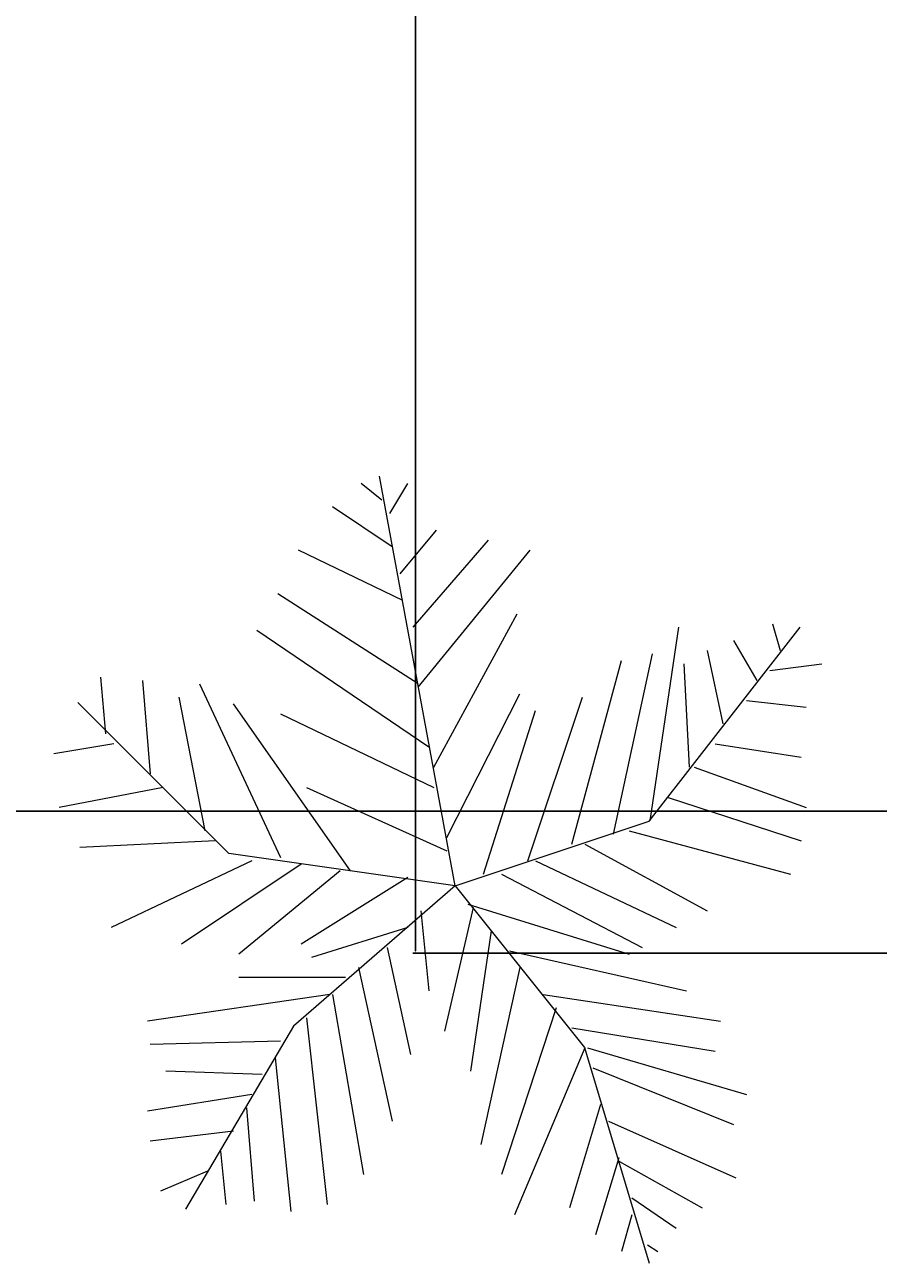
# Model space of a CAD drawing. Units: inches. Extents: x -301 to 715, y -607 to 364.
# Tile 92 of 141: x 134 to 194, y -256 to -168. Entities that reach past the tile are written whole.
import ezdxf

# ---------------------------------------------------------------- set-up
doc = ezdxf.new("R2010")
doc.units = ezdxf.units.IN
doc.header["$MEASUREMENT"] = 0
doc.layers.add('A-ANNO-DIMS', color=2, linetype='Continuous', lineweight=18)
doc.layers.add('L-PLNT', color=94, linetype='Continuous', lineweight=13)
doc.styles.get("Standard").update_dxf_attribs({"font": 'arial.ttf'})
doc.dimstyles.get("Standard").update_dxf_attribs({"dimtxt": 0.18, "dimasz": 0.18, "dimexe": 0.18, "dimexo": 0.0625, "dimgap": 0.09, "dimtad": 0, "dimtih": 1, "dimtoh": 1, "dimdec": 1, "dimzin": 0, "dimdsep": 46, "dimlunit": 4, "dimtxsty": 'Standard', "dimcen": 0.09, "dimclrd": 3, "dimclre": 4, "dimclrt": 6, "dimadec": 0, "dimazin": 0, "dimtfac": 1, "dimtdec": 1, "dimtofl": 0, "dimtmove": 0, "dimatfit": 3, "dimfxl": 1, "dimtfill": 2, "dimtfillclr": 51, "dimtolj": 1, "dimtzin": 0, "dimarcsym": 0})

# ---------------------------------------------------------------- blocks, each defined once
blk = doc.blocks.new('*U33')
for p, q in [((0, 0), (-10.5, 57)), ((-10.186, 53.64), (-13.084, 55.962)), ((-9.099, 51.782), (-6.563, 55.962)), ((-8.737, 47.138), (-17.069, 52.711)), ((-7.65, 43.423), (-2.578, 49.46)), ((-7.288, 39.707), (-21.778, 46.673)), ((-5.839, 35.992), (4.667, 48.067)), ((-5.114, 27.632), (10.463, 46.673)), ((-5.114, 28.097), (-24.676, 40.636)), ((-2.941, 16.486), (8.652, 37.85)), ((44.153, 36.456), (45.239, 32.741)), ((-3.665, 19.273), (-27.574, 35.527)), ((27, 9), (48, 36)), ((27.127, 9.056), (31.112, 35.992)), ((35.096, 32.741), (37.27, 22.524)), ((38.719, 34.134), (41.979, 28.561)), ((16.259, 5.805), (23.142, 31.348)), ((22.055, 7.198), (27.489, 32.277)), ((31.836, 30.883), (32.561, 16.486)), ((43.791, 29.954), (51.036, 30.883)), ((-48.585, 21.131), (-49.309, 29.026)), ((-43.513, 28.561), (-42.427, 15.558)), ((-35.544, 28.097), (-24.314, 3.947)), ((-38.442, 26.239), (-34.819, 7.663)), ((-1.129, 6.734), (9.014, 26.704)), ((10.101, 3.483), (17.708, 26.239)), ((-31.5, 4.5), (-52.5, 25.5)), ((-14.533, 2.09), (-30.834, 25.31)), ((3.942, 1.625), (11.187, 24.381)), ((40.53, 25.775), (48.862, 24.846)), ((-24.314, 23.917), (-2.941, 13.7)), ((-47.498, 19.737), (-55.83, 18.344)), ((36.183, 19.737), (48.137, 17.88)), ((33.285, 16.486), (48.862, 10.913)), ((-40.615, 13.7), (-55.105, 10.913)), ((-20.691, 13.7), (-1.129, 4.876)), ((29.662, 12.307), (48.137, 6.269)), ((0, 0), (27, 9)), ((24.229, 7.663), (46.688, 1.625)), ((-33.37, 6.269), (-52.207, 5.34)), ((18.07, 5.805), (35.096, -3.483)), ((-28.299, 3.483), (-47.86, -5.805)), ((0, 0), (-31.5, 4.5)), ((11.187, 3.483), (30.749, -5.805)), ((-21.416, 3.018), (-38.079, -8.128)), ((-15.982, 2.09), (-30.11, -9.521)), ((0, 0), (-22.5, -19.5)), ((-6.563, 1.161), (-21.416, -8.128)), ((0, 0), (18, -22.5)), ((6.478, 1.625), (26.04, -8.592)), ((2.493, -3.019), (-1.491, -20.202)), ((1.769, -2.555), (24.229, -9.521)), ((-4.752, -3.483), (-3.665, -14.629)), ((-6.563, -5.805), (-19.967, -9.985)), ((5.029, -6.27), (2.131, -25.775)), ((-9.461, -8.592), (-6.201, -23.453)), ((7.565, -9.056), (32.198, -14.629)), ((-13.446, -11.378), (-8.737, -32.741)), ((9.014, -11.378), (3.58, -35.992)), ((-15.257, -12.772), (-30.11, -12.772)), ((-17.431, -15.094), (-42.789, -18.809)), ((-17.069, -15.094), (-12.721, -40.172)), ((12.274, -15.094), (36.907, -18.809)), ((14.085, -16.951), (6.478, -40.172)), ((-20.691, -18.345), (-17.793, -44.352)), ((-22.5, -19.5), (-37.5, -45)), ((16.259, -19.738), (36.183, -22.989)), ((-24.314, -21.596), (-42.427, -22.06)), ((-25.038, -23.918), (-22.865, -45.281)), ((18.07, -22.524), (8.289, -45.745)), ((18, -22.5), (27, -52.5)), ((18.433, -22.524), (40.53, -29.026)), ((-26.849, -26.24), (-40.253, -25.775)), ((19.157, -25.311), (38.719, -33.206)), ((-28.299, -29.026), (-42.789, -31.348)), ((-29.023, -30.884), (-27.936, -43.887)), ((20.244, -30.419), (15.897, -44.816)), ((-30.834, -34.135), (-42.427, -35.528)), ((21.331, -32.741), (39.081, -40.636)), ((-32.646, -36.921), (-31.921, -44.352)), ((22.78, -37.85), (19.519, -48.532)), ((22.78, -38.314), (34.372, -44.816)), ((-34.457, -39.708), (-40.978, -42.494)), ((24.591, -43.423), (30.749, -47.603)), ((24.591, -45.745), (23.142, -50.854)), ((26.764, -49.925), (28.213, -50.854))]:
    blk.add_line(p, q)
blk = doc.blocks.new('*D152')
at = {"layer": 'A-ANNO-DIMS', "color": 4, "lineweight": -2, "transparency": 16777216}
for p, q in [((123.959, -130.818), (233.659, -130.818)), ((132.959, -223.818), (233.659, -223.818))]:
    blk.add_line(p, q, dxfattribs=at)
at = {"layer": 'A-ANNO-DIMS', "color": 3, "lineweight": -2, "transparency": 16777216}
for p, q in [((233.479, -130.998), (233.479, -177.136)), ((233.479, -223.638), (233.479, -177.5))]:
    blk.add_line(p, q, dxfattribs=at)
at = {"layer": 'A-ANNO-DIMS', "color": 3, "transparency": 16777216}
for points in [[(233.449, -130.998), (233.509, -130.998), (233.479, -130.818)], [(233.449, -223.638), (233.509, -223.638), (233.479, -223.818)]]:
    blk.add_solid(points, dxfattribs=at)
at = {"layer": 'Defpoints', "color": 0, "transparency": 16777216}
for p in [(123.897, -130.818), (233.479, -130.818), (132.897, -223.818)]:
    blk.add_point(p, dxfattribs=at)
at = {"layer": 'A-ANNO-DIMS', "color": 6, "transparency": 16777216, "insert": (233.479, -177.318), "char_height": 0.18, "attachment_point": 5, "bg_fill": 1, "box_fill_scale": 1.25, "bg_fill_color": 51, "bg_fill_transparency": 0}
blk.add_mtext('\\A1;7\'-9"', dxfattribs=at)
blk = doc.blocks.new('*D162')
at = {"layer": 'A-ANNO-DIMS', "color": 4, "lineweight": -2, "transparency": 16777216}
for p, q in [((222.328, 320.182), (161.439, 320.182)), ((222.328, -233.818), (161.439, -233.818))]:
    blk.add_line(p, q, dxfattribs=at)
at = {"layer": 'A-ANNO-DIMS', "color": 3, "lineweight": -2, "transparency": 16777216}
for p, q in [((161.619, 320.002), (161.619, 43.364)), ((161.619, -233.638), (161.619, 43))]:
    blk.add_line(p, q, dxfattribs=at)
at = {"layer": 'A-ANNO-DIMS', "color": 3, "transparency": 16777216}
for points in [[(161.589, 320.002), (161.649, 320.002), (161.619, 320.182)], [(161.589, -233.638), (161.649, -233.638), (161.619, -233.818)]]:
    blk.add_solid(points, dxfattribs=at)
at = {"layer": 'Defpoints', "color": 0, "transparency": 16777216}
for p in [(161.619, 320.182), (222.39, 320.182), (222.39, -233.818)]:
    blk.add_point(p, dxfattribs=at)
at = {"layer": 'A-ANNO-DIMS', "color": 6, "transparency": 16777216, "insert": (161.619, 43.182), "char_height": 0.18, "attachment_point": 5, "bg_fill": 1, "box_fill_scale": 1.25, "bg_fill_color": 51, "bg_fill_transparency": 0}
blk.add_mtext('\\A1;46\'-2"', dxfattribs=at)
blk = doc.blocks.new('*D167')
at = {"layer": 'A-ANNO-DIMS', "color": 4, "lineweight": -2, "transparency": 16777216}
for p, q in [((222.328, -83.318), (161.439, -83.318)), ((222.328, -233.818), (161.439, -233.818))]:
    blk.add_line(p, q, dxfattribs=at)
at = {"layer": 'A-ANNO-DIMS', "color": 3, "lineweight": -2, "transparency": 16777216}
for p, q in [((161.619, -83.498), (161.619, -158.385)), ((161.619, -233.638), (161.619, -158.751))]:
    blk.add_line(p, q, dxfattribs=at)
at = {"layer": 'A-ANNO-DIMS', "color": 3, "transparency": 16777216}
for points in [[(161.589, -83.498), (161.649, -83.498), (161.619, -83.318)], [(161.589, -233.638), (161.649, -233.638), (161.619, -233.818)]]:
    blk.add_solid(points, dxfattribs=at)
at = {"layer": 'Defpoints', "color": 0, "transparency": 16777216}
for p in [(161.619, -83.318), (222.39, -83.318), (222.39, -233.818)]:
    blk.add_point(p, dxfattribs=at)
at = {"layer": 'A-ANNO-DIMS', "color": 6, "transparency": 16777216, "insert": (161.619, -158.568), "char_height": 0.18, "attachment_point": 5, "bg_fill": 1, "box_fill_scale": 1.25, "bg_fill_color": 51, "bg_fill_transparency": 0}
blk.add_mtext('\\A1;12\'-6 1/2"', dxfattribs=at)

msp = doc.modelspace()

# ---------------------------------------------------------------- block references
at = {"layer": 'L-PLNT', "xscale": 0.5058896831792554, "yscale": 0.5058896831792554, "zscale": 0.5058896831792554}
msp.add_blockref('*U33', (164.406, -229.069), dxfattribs=at)

# ---------------------------------------------------------------- dimensions: what is measured, and where the dimension line sits
at = {"layer": 'A-ANNO-DIMS'}
for base, p1, p2, picture, middle in [((161.619, 320.182), (222.39, -233.818), (222.39, 320.182), '*D162', (161.619, 43.182)), ((161.619, -83.318), (222.39, -233.818), (222.39, -83.318), '*D167', (161.619, -158.568)), ((233.479, -130.818), (132.897, -223.818), (123.897, -130.818), '*D152', (233.479, -177.318))]:
    dim = msp.add_linear_dim(base=base, p1=p1, p2=p2, angle=90, dimstyle='Standard', override={"dimdec": 1, "dimlfac": 1, "dimrnd": 0, "dimzin": 1, "dimdsep": 46, "dimlunit": 4, "dimfrac": 2}, dxfattribs=at)
    dim.commit()
    dim.dimension.update_dxf_attribs({"geometry": picture, "text_midpoint": middle})

doc.saveas('drawing.dxf')
